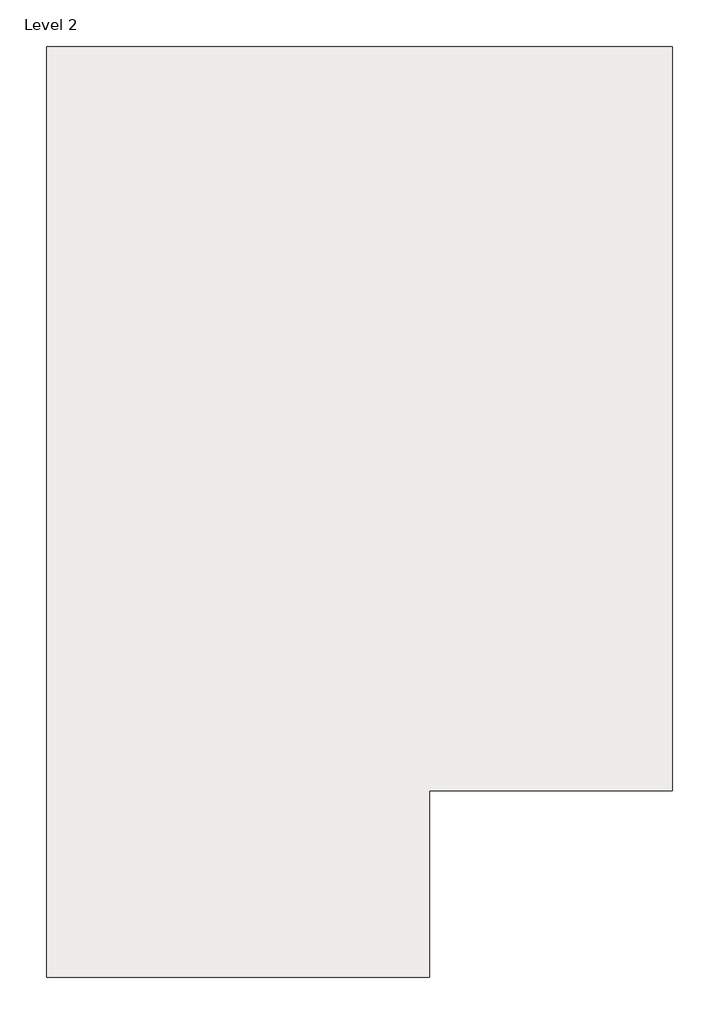
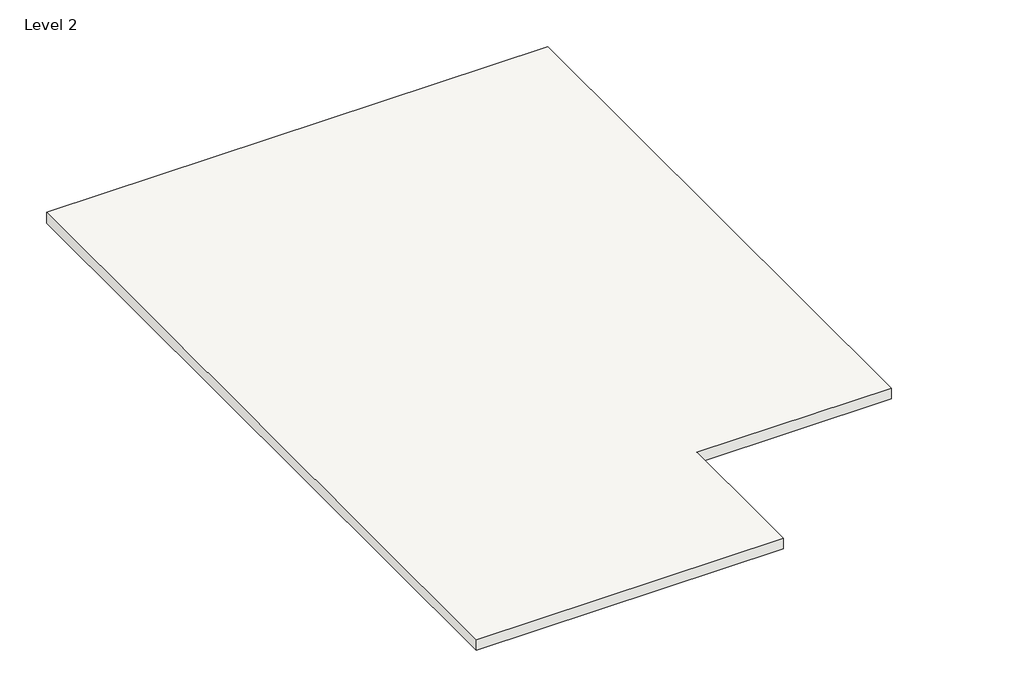
# One storey: 1 roof.
"""IFC4 building model written with IfcOpenShell, lengths in millimetres."""

from ifc_helpers import new_model, si_unit, frame, origin, place, context, project, spatial, polyline, outline, extrude, element, save

model = new_model("IFC4")

# Units and contexts
model_context = context("Model", 3, world=origin())
ifc_project = project(units=[si_unit("LENGTHUNIT", "METRE", prefix="MILLI")], contexts=[model_context])

# Site, building, storey
site = spatial("IfcSite", under=ifc_project)
building = spatial("IfcBuilding", under=site)
storey = spatial("IfcBuildingStorey", under=building, Name="Level 2", Elevation=3048.0)

# Roof
placement = place(None, origin())
element("IfcRoof", 1, ObjectType="Wood Rafter 8\" - Asphalt Shingle - Insulated", at=placement, inside=storey, context=model_context, shape_type="SweptSolid", body=[
    extrude(outline(polyline([(-14422.6389568, 15108.1342758), (-5126.2389568, 15108.1342758), (-5126.2389568, 4059.1342758), (-8733.0389568, 4059.1342758), (-8733.0389568, 2052.5342758), (-8733.0389568, 1290.5342758), (-14422.6389568, 1290.5342758), (-14422.6389568, 15108.1342758)])), frame((0.0, 0.0, 3048.0), z_axis=(0.0, 0.0, 1.0), x_axis=(1.0, 0.0, 0.0)), (0.0, 0.0, 1.0), 212.725),
])

save(model, "model.ifc")

# Revit data of these elements
# Type "Wood Rafter 8\" - Asphalt Shingle - Insulated"
#   Assembly Code = "B1020"
#   Layers, outside or top first: 0' - 0 1/4" "Asphalt Shingle" (function 4); 0' - 0 5/8" "Plywood, Sheathing" (function 2); 0' - 7 1/2" "Structure, Wood Joist/Rafter Layer, Batt Insulation" (function 1)
# Element 1 (IfcRoof, "Wood Rafter 8\" - Asphalt Shingle - Insulated")
#   built-in parameter 1001705 = 10.6979 (stored number, unit not read)
#   built-in parameter 1001710 = 33615
#   Phase Created = New Construction
#   Materials on its faces: "Structure, Wood Joist/Rafter Layer, Batt Insulation", "Asphalt Shingle"
# Materials
#   "Asphalt Shingle": class "Generic", colour RGB 155 155 155, transparency 0, Description = "Asphalt roofing shingle", Cost = 0
#   "Plywood, Sheathing": class "Wood", colour RGB 212 179 113, transparency 0, Description = "Plywood, sheathing grade", Cost = 0
#   "Structure, Wood Joist/Rafter Layer, Batt Insulation": class "Wood", colour RGB 127 127 127, transparency 0, Description = "Wood framing, insulated", Cost = 0
